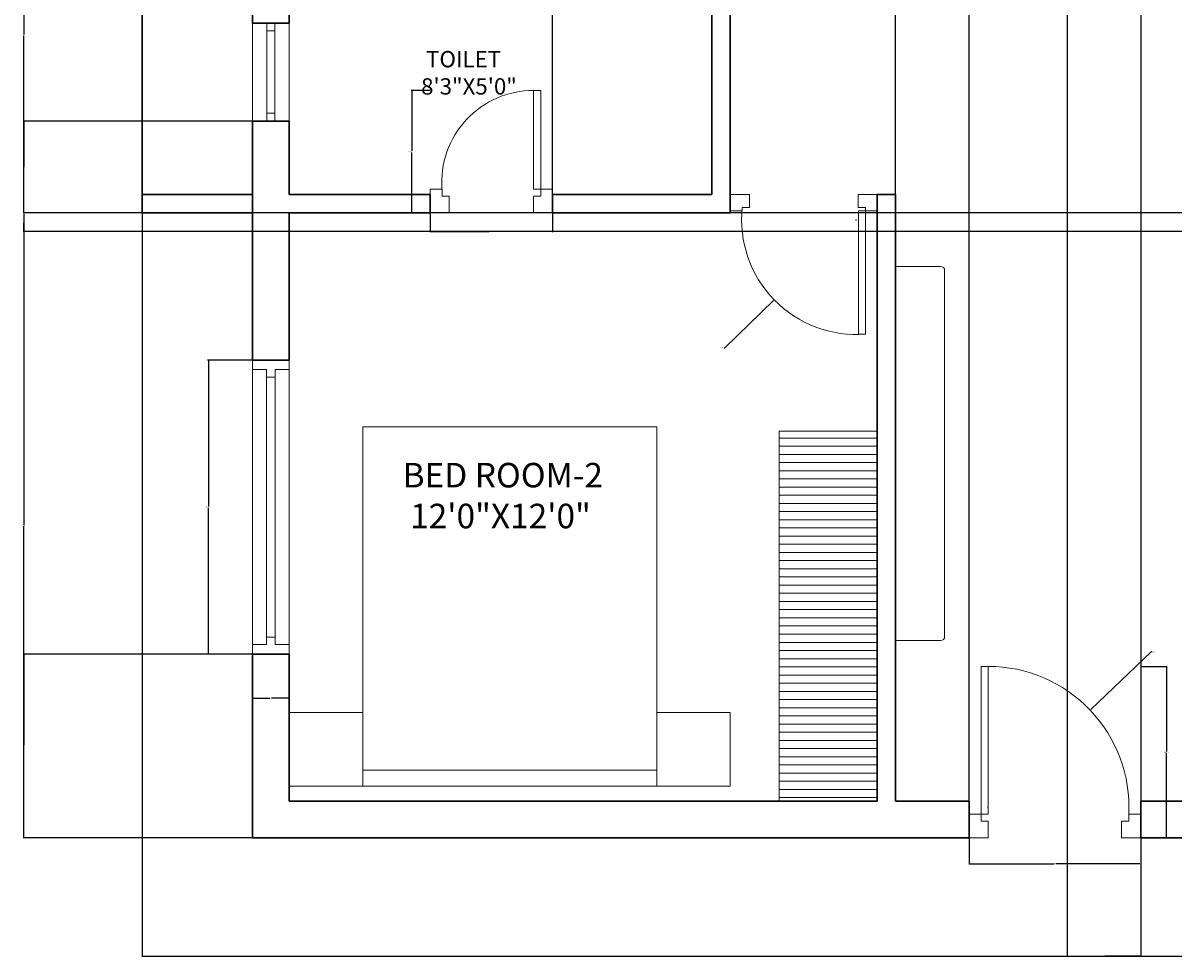
# Model space of a CAD drawing. Units: inches. Extents: x 2134 to 2768, y 715 to 1206.
# Tile 1 of 4: x 2135 to 2416, y 715 to 944. Entities that reach past the tile are written whole.
import ezdxf

# ---------------------------------------------------------------- set-up
doc = ezdxf.new("R2010")
doc.units = ezdxf.units.IN
for name, color, linetype, lineweight in [('A-ANNO-DIMS', 2, 'Continuous', 18), ('A-AREA-IDEN', 7, 'Continuous', 18), ('A-DOOR', 251, 'Continuous', 13), ('A-FLOR-CASE', 251, 'Continuous', 13), ('A-FLOR-CASE-PATT', 252, 'Continuous', 9), ('A-FURN', 251, 'Continuous', 13), ('A-WALL', 7, 'Continuous', 30), ('A-WINDOW', 251, 'Continuous', 13)]:
    doc.layers.add(name, color=color, linetype=linetype, lineweight=lineweight)
doc.styles.get("Standard").update_dxf_attribs({"font": 'arial.ttf'})
doc.dimstyles.get("Standard").update_dxf_attribs({"dimtxt": 0.18, "dimasz": 0.18, "dimexe": 0.18, "dimexo": 0.0625, "dimgap": 0.09, "dimtad": 0, "dimtih": 1, "dimtoh": 1, "dimdec": 4, "dimzin": 0, "dimdsep": 46, "dimtxsty": 'Standard', "dimcen": 0.09, "dimadec": 0, "dimazin": 0, "dimtfac": 1, "dimtdec": 4, "dimtofl": 0, "dimtmove": 0, "dimatfit": 3, "dimfxl": 1, "dimtolj": 1, "dimtzin": 0, "dimarcsym": 0})

# ---------------------------------------------------------------- blocks, each defined once
blk = doc.blocks.new('3 6 2')
at = {"layer": 'A-DOOR'}
for points in [[(-36.75, 5.83), (-36.75, 42), (-35, 42), (-35, 5.83)], [(-36.75, 4.08), (-35, 4.08), (-35, 0), (-39.67, 0), (-39.67, 5.83), (-36.75, 5.83)], [(-0.58, 5.83), (-0.58, 4.08), (-2.33, 4.08), (-2.33, 0), (2.33, 0), (2.33, 5.83)]]:
    blk.add_lwpolyline(points, close=True, dxfattribs=at)
at = {"layer": 'A-DOOR', "ltscale": 0.1}
blk.add_arc((-35, 7.54), 34.46, 357.1595, 90, dxfattribs=at)
blk = doc.blocks.new('ARCHITRAVE')
at = {"layer": 'A-DOOR'}
for p, q in [((0, 0), (0, 4)), ((0, 3.99), (2.92, 3.99)), ((2.92, 3.99), (2.92, 3.17)), ((2.92, 3.17), (4.67, 3.17)), ((4.67, 3.17), (4.67, 0)), ((4.67, 0), (0, 0))]:
    blk.add_line(p, q, dxfattribs=at)
blk = doc.blocks.new('3 FEET DOOR')
at = {"layer": 'A-DOOR'}
blk.add_lwpolyline([(-34.02, 3.98), (-34.02, 34.15), (-32.27, 34.15), (-32.27, 3.98)], close=True, dxfattribs=at)
at = {"layer": 'A-DOOR', "ltscale": 0.1}
blk.add_arc((-31.74, 6.19), 28.05, 353.8214, 94.662, dxfattribs=at)
at = {"layer": 'A-DOOR'}
blk.add_blockref('ARCHITRAVE', (-36.91, 0), dxfattribs=at)
at = {"layer": 'A-DOOR', "xscale": -1}
blk.add_blockref('ARCHITRAVE', (-0.93, 0), dxfattribs=at)
blk = doc.blocks.new('2 feet 6 inch door')
at = {"layer": 'A-DOOR'}
for points in [[(2.92, 5.83), (2.92, 30), (4.67, 30), (4.67, 5.83)], [(2.92, 4.08), (4.67, 4.08), (4.67, 0), (0, 0), (0, 5.83), (2.92, 5.83)], [(27.08, 5.83), (27.08, 4.08), (25.33, 4.08), (25.33, 0), (30, 0), (30, 5.83)]]:
    blk.add_lwpolyline(points, close=True, dxfattribs=at)
at = {"layer": 'A-DOOR', "ltscale": 0.1}
blk.add_arc((4.67, 7.52), 22.48, 355.6972, 90, dxfattribs=at)
blk = doc.blocks.new('bed')
at = {"layer": 'A-FURN'}
for points in [[(3369.68, 925.24), (3297.68, 925.24), (3297.68, 1009.24), (3369.68, 1009.24)], [(3297.68, 921.32), (3279.68, 921.32), (3279.68, 939.32), (3297.68, 939.32)], [(3369.68, 921.32), (3387.68, 921.32), (3387.68, 939.32), (3369.68, 939.32)], [(3297.68, 925.24), (3369.68, 925.24), (3369.68, 921.32), (3297.68, 921.32)]]:
    blk.add_lwpolyline(points, close=True, dxfattribs=at)
blk = doc.blocks.new("2' ventilators")
at = {"layer": 'A-WINDOW'}
for p, q in [((24, 5.5), (0, 5.5)), ((1.93, 5.5), (1.93, 3.5)), ((22.07, 5.5), (22.07, 3.5))]:
    blk.add_line(p, q, dxfattribs=at)
for points in [[(0, 9), (24, 9), (24, 0), (0, 0), (0, 9)], [(24, 3.5), (0, 3.5)]]:
    blk.add_lwpolyline(points, dxfattribs=at)
blk = doc.blocks.new('WINDOW FRAME')
at = {"layer": 'A-WINDOW'}
for points in [[(4178.2, 4970.76), (4174.8, 4970.76), (4174.8, 4968.41), (4183.8, 4968.41), (4183.8, 4970.76), (4180.39, 4970.76)], [(4180.39, 4970.76), (4180.39, 4972.59), (4178.2, 4972.59), (4178.2, 4970.76)]]:
    blk.add_lwpolyline(points, dxfattribs=at)
blk = doc.blocks.new('6 feet door')
at = {"layer": 'A-WINDOW'}
for p, q in [((-69.65, 9), (-2.35, 9)), ((-4.18, 5.59), (-67.82, 5.59)), ((-4.18, 3.41), (-67.82, 3.41)), ((-69.65, 0), (-2.35, 0))]:
    blk.add_line(p, q, dxfattribs=at)
at = {"layer": 'A-WINDOW', "rotation": 270}
blk.add_blockref('WINDOW FRAME', (-5040.41, 4183.8), dxfattribs=at)
at = {"layer": 'A-WINDOW', "xscale": -1, "rotation": 90}
blk.add_blockref('WINDOW FRAME', (4968.41, 4183.8), dxfattribs=at)
blk = doc.blocks.new('*D53')
at = {"layer": 'A-ANNO-DIMS', "color": 0, "lineweight": -2, "transparency": 16777216}
for p, q in [((2234.22, 927.11), (2229.61, 927.11)), ((2229.79, 926.93), (2229.79, 912.29)), ((2229.79, 897.29), (2229.79, 911.92)), ((2234.22, 897.11), (2229.61, 897.11))]:
    blk.add_line(p, q, dxfattribs=at)
at = {"layer": 'A-ANNO-DIMS', "color": 0, "transparency": 16777216}
for points in [[(2229.76, 926.93), (2229.82, 926.93), (2229.79, 927.11)], [(2229.76, 897.29), (2229.82, 897.29), (2229.79, 897.11)]]:
    blk.add_solid(points, dxfattribs=at)
at = {"layer": 'Defpoints', "color": 0, "transparency": 16777216}
for p in [(2229.79, 927.11), (2234.29, 927.11), (2234.29, 897.11)]:
    blk.add_point(p, dxfattribs=at)
at = {"layer": 'A-ANNO-DIMS', "color": 0, "transparency": 16777216, "insert": (2229.79, 912.11), "char_height": 0.18, "attachment_point": 5}
blk.add_mtext('\\A1;BATH DOOR 30 TYP.', dxfattribs=at)
blk = doc.blocks.new('*D54')
at = {"layer": 'A-ANNO-DIMS', "color": 0, "lineweight": -2, "transparency": 16777216}
for p, q in [((2234.29, 897.04), (2234.29, 892.43)), ((2264.29, 897.04), (2264.29, 892.43)), ((2234.47, 892.61), (2248.76, 892.61)), ((2264.11, 892.61), (2249.82, 892.61))]:
    blk.add_line(p, q, dxfattribs=at)
at = {"layer": 'A-ANNO-DIMS', "color": 0, "transparency": 16777216}
for points in [[(2234.47, 892.64), (2234.47, 892.58), (2234.29, 892.61)], [(2264.11, 892.64), (2264.11, 892.58), (2264.29, 892.61)]]:
    blk.add_solid(points, dxfattribs=at)
at = {"layer": 'Defpoints', "color": 0, "transparency": 16777216}
for p in [(2234.29, 897.11), (2264.29, 897.11), (2234.29, 892.61)]:
    blk.add_point(p, dxfattribs=at)
at = {"layer": 'A-ANNO-DIMS', "color": 0, "transparency": 16777216, "insert": (2249.29, 892.61), "char_height": 0.18, "attachment_point": 5}
blk.add_mtext('\\A1;30 TYP.', dxfattribs=at)
blk = doc.blocks.new('*D69')
at = {"layer": 'A-ANNO-DIMS', "color": 0, "lineweight": -2, "transparency": 16777216}
for p, q in [((2408.35, 786.11), (2414.77, 786.11)), ((2414.59, 785.93), (2414.59, 765.29)), ((2414.59, 744.29), (2414.59, 764.93)), ((2408.35, 744.11), (2414.77, 744.11))]:
    blk.add_line(p, q, dxfattribs=at)
at = {"layer": 'A-ANNO-DIMS', "color": 0, "transparency": 16777216}
for points in [[(2414.56, 785.93), (2414.62, 785.93), (2414.59, 786.11)], [(2414.56, 744.29), (2414.62, 744.29), (2414.59, 744.11)]]:
    blk.add_solid(points, dxfattribs=at)
at = {"layer": 'Defpoints', "color": 0, "transparency": 16777216}
for p in [(2408.29, 786.11), (2414.59, 786.11), (2408.29, 744.11)]:
    blk.add_point(p, dxfattribs=at)
at = {"layer": 'A-ANNO-DIMS', "color": 0, "transparency": 16777216, "insert": (2414.59, 765.11), "char_height": 0.18, "attachment_point": 5}
blk.add_mtext('\\A1;ENTRY 42', dxfattribs=at)
blk = doc.blocks.new('*D70')
at = {"layer": 'A-ANNO-DIMS', "color": 0, "lineweight": -2, "transparency": 16777216}
for p, q in [((2366.29, 744.04), (2366.29, 737.63)), ((2408.29, 744.04), (2408.29, 737.63)), ((2366.47, 737.81), (2387.07, 737.81)), ((2408.11, 737.81), (2387.51, 737.81))]:
    blk.add_line(p, q, dxfattribs=at)
at = {"layer": 'A-ANNO-DIMS', "color": 0, "transparency": 16777216}
for points in [[(2366.47, 737.84), (2366.47, 737.78), (2366.29, 737.81)], [(2408.11, 737.84), (2408.11, 737.78), (2408.29, 737.81)]]:
    blk.add_solid(points, dxfattribs=at)
at = {"layer": 'Defpoints', "color": 0, "transparency": 16777216}
for p in [(2366.29, 744.11), (2408.29, 744.11), (2408.29, 737.81)]:
    blk.add_point(p, dxfattribs=at)
at = {"layer": 'A-ANNO-DIMS', "color": 0, "transparency": 16777216, "insert": (2387.29, 737.81), "char_height": 0.18, "attachment_point": 5}
blk.add_mtext('\\A1;42', dxfattribs=at)
blk = doc.blocks.new('*D73')
at = {"layer": 'A-ANNO-DIMS', "color": 0, "lineweight": -2, "transparency": 16777216}
for p, q in [((2190.72, 861.11), (2179.81, 861.11)), ((2179.99, 860.93), (2179.99, 825.29)), ((2179.99, 789.29), (2179.99, 824.92)), ((2190.72, 789.11), (2179.81, 789.11))]:
    blk.add_line(p, q, dxfattribs=at)
at = {"layer": 'A-ANNO-DIMS', "color": 0, "transparency": 16777216}
for points in [[(2179.96, 860.93), (2180.02, 860.93), (2179.99, 861.11)], [(2179.96, 789.29), (2180.02, 789.29), (2179.99, 789.11)]]:
    blk.add_solid(points, dxfattribs=at)
at = {"layer": 'Defpoints', "color": 0, "transparency": 16777216}
for p in [(2190.79, 861.11), (2179.99, 789.11), (2190.79, 789.11)]:
    blk.add_point(p, dxfattribs=at)
at = {"layer": 'A-ANNO-DIMS', "color": 0, "transparency": 16777216, "insert": (2179.99, 825.11), "char_height": 0.18, "attachment_point": 5}
blk.add_mtext('\\A1;GLAZING 72', dxfattribs=at)
blk = doc.blocks.new('*D74')
at = {"layer": 'A-ANNO-DIMS', "color": 0, "lineweight": -2, "transparency": 16777216}
for p, q in [((2190.79, 789.04), (2190.79, 778.13)), ((2199.79, 789.04), (2199.79, 778.13)), ((2190.97, 778.31), (2195.14, 778.31)), ((2199.61, 778.31), (2195.44, 778.31))]:
    blk.add_line(p, q, dxfattribs=at)
at = {"layer": 'A-ANNO-DIMS', "color": 0, "transparency": 16777216}
for points in [[(2190.97, 778.34), (2190.97, 778.28), (2190.79, 778.31)], [(2199.61, 778.34), (2199.61, 778.28), (2199.79, 778.31)]]:
    blk.add_solid(points, dxfattribs=at)
at = {"layer": 'Defpoints', "color": 0, "transparency": 16777216}
for p in [(2190.79, 789.11), (2199.79, 789.11), (2199.79, 778.31)]:
    blk.add_point(p, dxfattribs=at)
at = {"layer": 'A-ANNO-DIMS', "color": 0, "transparency": 16777216, "insert": (2195.29, 778.31), "char_height": 0.18, "attachment_point": 5}
blk.add_mtext('\\A1;9', dxfattribs=at)
blk = doc.blocks.new('*D81')
at = {"layer": 'A-ANNO-DIMS', "color": 0, "lineweight": -2, "transparency": 16777216}
for p, q in [((2163.72, 897.11), (2134.66, 897.11)), ((2134.84, 896.93), (2134.84, 820.79)), ((2134.84, 744.29), (2134.84, 820.43)), ((2190.72, 744.11), (2134.66, 744.11))]:
    blk.add_line(p, q, dxfattribs=at)
at = {"layer": 'A-ANNO-DIMS', "color": 0, "transparency": 16777216}
for points in [[(2134.81, 896.93), (2134.87, 896.93), (2134.84, 897.11)], [(2134.81, 744.29), (2134.87, 744.29), (2134.84, 744.11)]]:
    blk.add_solid(points, dxfattribs=at)
at = {"layer": 'Defpoints', "color": 0, "transparency": 16777216}
for p in [(2134.84, 897.11), (2163.79, 897.11), (2190.79, 744.11)]:
    blk.add_point(p, dxfattribs=at)
at = {"layer": 'A-ANNO-DIMS', "color": 0, "transparency": 16777216, "insert": (2134.84, 820.61), "char_height": 0.18, "attachment_point": 5}
blk.add_mtext('\\A1;153', dxfattribs=at)
blk = doc.blocks.new('*D82')
at = {"layer": 'A-ANNO-DIMS', "color": 0, "lineweight": -2, "transparency": 16777216}
for p, q in [((2163.72, 984.11), (2134.66, 984.11)), ((2134.84, 983.93), (2134.84, 940.79)), ((2134.84, 897.29), (2134.84, 940.43)), ((2163.72, 897.11), (2134.66, 897.11))]:
    blk.add_line(p, q, dxfattribs=at)
at = {"layer": 'A-ANNO-DIMS', "color": 0, "transparency": 16777216}
for points in [[(2134.81, 983.93), (2134.87, 983.93), (2134.84, 984.11)], [(2134.81, 897.29), (2134.87, 897.29), (2134.84, 897.11)]]:
    blk.add_solid(points, dxfattribs=at)
at = {"layer": 'Defpoints', "color": 0, "transparency": 16777216}
for p in [(2134.84, 984.11), (2163.79, 984.11), (2163.79, 897.11)]:
    blk.add_point(p, dxfattribs=at)
at = {"layer": 'A-ANNO-DIMS', "color": 0, "transparency": 16777216, "insert": (2134.84, 940.61), "char_height": 0.18, "attachment_point": 5}
blk.add_mtext('\\A1;87', dxfattribs=at)
blk = doc.blocks.new('*D83')
at = {"layer": 'A-ANNO-DIMS', "color": 0, "lineweight": -2, "transparency": 16777216}
for p, q in [((2348.29, 753.17), (2348.29, 1205.74)), ((2348.47, 1205.56), (2357.08, 1205.56)), ((2366.11, 1205.56), (2357.5, 1205.56)), ((2366.29, 753.17), (2366.29, 1205.74))]:
    blk.add_line(p, q, dxfattribs=at)
at = {"layer": 'A-ANNO-DIMS', "color": 0, "transparency": 16777216}
for points in [[(2348.47, 1205.59), (2348.47, 1205.53), (2348.29, 1205.56)], [(2366.11, 1205.59), (2366.11, 1205.53), (2366.29, 1205.56)]]:
    blk.add_solid(points, dxfattribs=at)
at = {"layer": 'Defpoints', "color": 0, "transparency": 16777216}
for p in [(2366.29, 1205.56), (2348.29, 753.11), (2366.29, 753.11)]:
    blk.add_point(p, dxfattribs=at)
at = {"layer": 'A-ANNO-DIMS', "color": 0, "transparency": 16777216, "insert": (2357.29, 1205.56), "char_height": 0.18, "attachment_point": 5}
blk.add_mtext('\\A1;18', dxfattribs=at)
blk = doc.blocks.new('*D86')
at = {"layer": 'A-ANNO-DIMS', "color": 0, "lineweight": -2, "transparency": 16777216}
for p, q in [((2190.72, 789.11), (2134.66, 789.11)), ((2134.84, 788.93), (2134.84, 766.79)), ((2134.84, 744.29), (2134.84, 766.43)), ((2190.72, 744.11), (2134.66, 744.11))]:
    blk.add_line(p, q, dxfattribs=at)
at = {"layer": 'A-ANNO-DIMS', "color": 0, "transparency": 16777216}
for points in [[(2134.81, 788.93), (2134.87, 788.93), (2134.84, 789.11)], [(2134.81, 744.29), (2134.87, 744.29), (2134.84, 744.11)]]:
    blk.add_solid(points, dxfattribs=at)
at = {"layer": 'Defpoints', "color": 0, "transparency": 16777216}
for p in [(2134.84, 789.11), (2190.79, 789.11), (2190.79, 744.11)]:
    blk.add_point(p, dxfattribs=at)
at = {"layer": 'A-ANNO-DIMS', "color": 0, "transparency": 16777216, "insert": (2134.84, 766.61), "char_height": 0.18, "attachment_point": 5}
blk.add_mtext('\\A1;45', dxfattribs=at)
blk = doc.blocks.new('*D88')
at = {"layer": 'A-ANNO-DIMS', "color": 0, "lineweight": -2, "transparency": 16777216}
for p, q in [((2190.72, 919.61), (2134.66, 919.61)), ((2134.84, 919.43), (2134.84, 908.54)), ((2134.84, 897.29), (2134.84, 908.18)), ((2190.72, 897.11), (2134.66, 897.11))]:
    blk.add_line(p, q, dxfattribs=at)
at = {"layer": 'A-ANNO-DIMS', "color": 0, "transparency": 16777216}
for points in [[(2134.81, 919.43), (2134.87, 919.43), (2134.84, 919.61)], [(2134.81, 897.29), (2134.87, 897.29), (2134.84, 897.11)]]:
    blk.add_solid(points, dxfattribs=at)
at = {"layer": 'Defpoints', "color": 0, "transparency": 16777216}
for p in [(2134.84, 919.61), (2190.79, 919.61), (2190.79, 897.11)]:
    blk.add_point(p, dxfattribs=at)
at = {"layer": 'A-ANNO-DIMS', "color": 0, "transparency": 16777216, "insert": (2134.84, 908.36), "char_height": 0.18, "attachment_point": 5}
blk.add_mtext('\\A1;22.5', dxfattribs=at)
blk = doc.blocks.new('*D90')
at = {"layer": 'A-ANNO-DIMS', "color": 0, "lineweight": -2, "transparency": 16777216}
for p, q in [((2729.72, 897.11), (2134.66, 897.11)), ((2134.84, 896.93), (2134.84, 895.04)), ((2134.84, 892.79), (2134.84, 894.68)), ((2729.72, 892.61), (2134.66, 892.61))]:
    blk.add_line(p, q, dxfattribs=at)
at = {"layer": 'A-ANNO-DIMS', "color": 0, "transparency": 16777216}
for points in [[(2134.81, 896.93), (2134.87, 896.93), (2134.84, 897.11)], [(2134.81, 892.79), (2134.87, 892.79), (2134.84, 892.61)]]:
    blk.add_solid(points, dxfattribs=at)
at = {"layer": 'Defpoints', "color": 0, "transparency": 16777216}
for p in [(2729.79, 897.11), (2134.84, 892.61), (2729.79, 892.61)]:
    blk.add_point(p, dxfattribs=at)
at = {"layer": 'A-ANNO-DIMS', "color": 0, "transparency": 16777216, "insert": (2134.84, 894.86), "char_height": 0.18, "attachment_point": 5}
blk.add_mtext('\\A1;4.5', dxfattribs=at)
blk = doc.blocks.new('*D91')
at = {"layer": 'A-ANNO-DIMS', "color": 0, "lineweight": -2, "transparency": 16777216}
for p, q in [((2390.29, 1115.04), (2390.29, 714.98)), ((2408.29, 1115.04), (2408.29, 714.98)), ((2390.47, 715.16), (2399.08, 715.16)), ((2408.11, 715.16), (2399.5, 715.16))]:
    blk.add_line(p, q, dxfattribs=at)
at = {"layer": 'A-ANNO-DIMS', "color": 0, "transparency": 16777216}
for points in [[(2390.47, 715.19), (2390.47, 715.13), (2390.29, 715.16)], [(2408.11, 715.19), (2408.11, 715.13), (2408.29, 715.16)]]:
    blk.add_solid(points, dxfattribs=at)
at = {"layer": 'Defpoints', "color": 0, "transparency": 16777216}
for p in [(2390.29, 1115.11), (2408.29, 1115.11), (2408.29, 715.16)]:
    blk.add_point(p, dxfattribs=at)
at = {"layer": 'A-ANNO-DIMS', "color": 0, "transparency": 16777216, "insert": (2399.29, 715.16), "char_height": 0.18, "attachment_point": 5}
blk.add_mtext('\\A1;18', dxfattribs=at)
blk = doc.blocks.new('*D103')
at = {"layer": 'A-ANNO-DIMS', "color": 0, "lineweight": -2, "transparency": 16777216}
for p, q in [((2264.29, 901.67), (2264.29, 1205.74)), ((2264.47, 1205.56), (2283.57, 1205.56)), ((2303.11, 1205.56), (2284.01, 1205.56)), ((2303.29, 901.67), (2303.29, 1205.74))]:
    blk.add_line(p, q, dxfattribs=at)
at = {"layer": 'A-ANNO-DIMS', "color": 0, "transparency": 16777216}
for points in [[(2264.47, 1205.59), (2264.47, 1205.53), (2264.29, 1205.56)], [(2303.11, 1205.59), (2303.11, 1205.53), (2303.29, 1205.56)]]:
    blk.add_solid(points, dxfattribs=at)
at = {"layer": 'Defpoints', "color": 0, "transparency": 16777216}
for p in [(2303.29, 1205.56), (2264.29, 901.61), (2303.29, 901.61)]:
    blk.add_point(p, dxfattribs=at)
at = {"layer": 'A-ANNO-DIMS', "color": 0, "transparency": 16777216, "insert": (2283.79, 1205.56), "char_height": 0.18, "attachment_point": 5}
blk.add_mtext('\\A1;39', dxfattribs=at)
blk = doc.blocks.new('*D105')
at = {"layer": 'A-ANNO-DIMS', "color": 0, "lineweight": -2, "transparency": 16777216}
for p, q in [((2163.79, 897.04), (2163.79, 714.98)), ((2738.79, 744.04), (2738.79, 714.98)), ((2163.97, 715.16), (2451, 715.16)), ((2738.61, 715.16), (2451.58, 715.16))]:
    blk.add_line(p, q, dxfattribs=at)
at = {"layer": 'A-ANNO-DIMS', "color": 0, "transparency": 16777216}
for points in [[(2163.97, 715.19), (2163.97, 715.13), (2163.79, 715.16)], [(2738.61, 715.19), (2738.61, 715.13), (2738.79, 715.16)]]:
    blk.add_solid(points, dxfattribs=at)
at = {"layer": 'Defpoints', "color": 0, "transparency": 16777216}
for p in [(2163.79, 897.11), (2738.79, 744.11), (2738.79, 715.16)]:
    blk.add_point(p, dxfattribs=at)
at = {"layer": 'A-ANNO-DIMS', "color": 0, "transparency": 16777216, "insert": (2451.29, 715.16), "char_height": 0.18, "attachment_point": 5}
blk.add_mtext('\\A1;575', dxfattribs=at)
blk = doc.blocks.new('*D107')
at = {"layer": 'A-ANNO-DIMS', "color": 0, "lineweight": -2, "transparency": 16777216}
for p, q in [((2410.89, 789.66), (2396.05, 775.53)), ((2411.07, 789.66), (2410.89, 789.66)), ((2370.86, 751.65), (2371.04, 751.65)), ((2370.95, 751.56), (2370.95, 751.74))]:
    blk.add_line(p, q, dxfattribs=at)
at = {"layer": 'A-ANNO-DIMS', "color": 0, "transparency": 16777216}
blk.add_solid([(2396.03, 775.55), (2396.07, 775.51), (2395.92, 775.4)], dxfattribs=at)
at = {"layer": 'Defpoints', "color": 0, "transparency": 16777216}
for p in [(2395.92, 775.4), (2370.95, 751.65)]:
    blk.add_point(p, dxfattribs=at)
at = {"layer": 'A-ANNO-DIMS', "color": 0, "transparency": 16777216, "insert": (2411.55, 789.66), "char_height": 0.18, "attachment_point": 5}
blk.add_mtext('\\A1;R34.46', dxfattribs=at)
blk = doc.blocks.new('*D108')
at = {"layer": 'A-ANNO-DIMS', "color": 0, "lineweight": -2, "transparency": 16777216}
for p, q in [((2338.62, 895.33), (2338.62, 895.51)), ((2338.53, 895.42), (2338.71, 895.42)), ((2306.47, 864.1), (2318.39, 875.72)), ((2306.29, 864.1), (2306.47, 864.1))]:
    blk.add_line(p, q, dxfattribs=at)
at = {"layer": 'A-ANNO-DIMS', "color": 0, "transparency": 16777216}
blk.add_solid([(2318.37, 875.74), (2318.42, 875.7), (2318.52, 875.85)], dxfattribs=at)
at = {"layer": 'Defpoints', "color": 0, "transparency": 16777216}
for p in [(2338.62, 895.42), (2318.52, 875.85)]:
    blk.add_point(p, dxfattribs=at)
at = {"layer": 'A-ANNO-DIMS', "color": 0, "transparency": 16777216, "insert": (2305.81, 864.1), "char_height": 0.18, "attachment_point": 5}
blk.add_mtext('\\A1;R28.05', dxfattribs=at)

msp = doc.modelspace()

# ---------------------------------------------------------------- hatches: boundary and pattern name
at = {"layer": 'A-FLOR-CASE-PATT'}
h = msp.add_hatch(dxfattribs=at)
h.set_pattern_fill('_USER', color=256, scale=2, pattern_type=0)
h.set_pattern_definition([(0, (0, 0), (0, 2), [])])
h.paths.add_polyline_path([(2343.787, 843.68), (2319.787, 843.68), (2319.787, 753.107), (2343.787, 753.107)])

# ---------------------------------------------------------------- linework, layer by layer
at = {"layer": 'A-FLOR-CASE'}
for p, q in [((2348.287, 884.029), (2359.287, 884.029)), ((2360.287, 883.029), (2360.287, 793.422)), ((2319.787, 843.68), (2319.787, 753.107)), ((2319.787, 843.68), (2343.787, 843.68)), ((2359.287, 792.422), (2348.287, 792.422))]:
    msp.add_line(p, q, dxfattribs=at)
for centre, start, end in [((2359.287, 883.029), 0, 90), ((2359.287, 793.422), 270, 0)]:
    msp.add_arc(centre, 1, start, end, dxfattribs=at)
at = {"layer": 'A-WALL'}
for p, q in [((2163.787, 979.607), (2163.787, 901.607)), ((2190.787, 979.607), (2190.787, 943.607)), ((2307.787, 966.107), (2307.787, 897.107)), ((2199.787, 961.607), (2199.787, 943.607)), ((2303.287, 961.607), (2303.287, 901.607)), ((2199.787, 943.607), (2190.787, 943.607)), ((2199.787, 919.607), (2190.787, 919.607)), ((2190.787, 919.607), (2190.787, 861.107)), ((2199.787, 919.607), (2199.787, 901.607)), ((2163.787, 897.107), (2163.787, 901.607)), ((2190.787, 901.607), (2163.787, 901.607)), ((2234.287, 901.607), (2199.787, 901.607)), ((2234.287, 901.607), (2234.287, 897.107)), ((2303.287, 901.607), (2264.287, 901.607)), ((2264.287, 901.607), (2264.287, 897.107)), ((2343.787, 901.607), (2348.287, 901.607)), ((2343.787, 901.607), (2343.787, 753.107)), ((2348.287, 901.607), (2348.287, 753.107)), ((2190.787, 897.107), (2163.787, 897.107)), ((2234.287, 897.107), (2199.787, 897.107)), ((2199.787, 897.107), (2199.787, 861.107)), ((2307.787, 897.107), (2264.287, 897.107)), ((2199.787, 861.107), (2190.787, 861.107)), ((2199.787, 789.107), (2190.787, 789.107)), ((2190.787, 789.107), (2190.787, 744.107)), ((2199.787, 789.107), (2199.787, 753.107)), ((2343.787, 753.107), (2199.787, 753.107)), ((2366.287, 753.107), (2348.287, 753.107)), ((2366.287, 753.107), (2366.287, 744.107)), ((2408.287, 753.107), (2408.287, 744.107)), ((2467.287, 753.107), (2408.287, 753.107)), ((2366.287, 744.107), (2190.787, 744.107)), ((2467.287, 744.107), (2408.287, 744.107))]:
    msp.add_line(p, q, dxfattribs=at)

# ---------------------------------------------------------------- block references
at = {"layer": 'A-DOOR', "xscale": -1}
msp.add_blockref('2 feet 6 inch door', (2264.287, 897.107), dxfattribs=at)
at = {"layer": 'A-DOOR', "rotation": 180}
msp.add_blockref('3 FEET DOOR', (2306.88, 901.607), dxfattribs=at)
at = {"layer": 'A-DOOR'}
msp.add_blockref('3 6 2', (2405.954, 744.107), dxfattribs=at)
at = {"layer": 'A-FURN'}
msp.add_blockref('bed', (-1079.895, -164.514), dxfattribs=at)
at = {"layer": 'A-WINDOW'}
for name, p, rotation in [("2' ventilators", (2190.787, 943.607), 270), ('6 feet door', (2190.787, 789.107), 270.000009980655)]:
    msp.add_blockref(name, p, dxfattribs=dict(at, rotation=rotation))

# ---------------------------------------------------------------- texts
at = {"layer": 'A-AREA-IDEN', "attachment_point": 1}
for s, insert, char_height in [('  TOILET\\P 8\'3"X5\'0"', (2230.859, 936.756), 4), ('BED ROOM-2\\P 12\'0"X12\'0"', (2227.563, 835.925), 6)]:
    msp.add_mtext_dynamic_manual_height_columns(s, width=55.72169, gutter_width=12.5, heights=[0], dxfattribs=dict(at, insert=insert, char_height=char_height))

# ---------------------------------------------------------------- dimensions: what is measured, and where the dimension line sits
at = {"layer": 'A-ANNO-DIMS'}
for base, p1, p2, picture, middle in [((2303.287, 1205.557), (2264.287, 901.607), (2303.287, 901.607), '*D103', (2283.787, 1205.557)), ((2366.287, 1205.557), (2348.287, 753.107), (2366.287, 753.107), '*D83', (2357.287, 1205.557)), ((2408.287, 715.157), (2390.287, 1115.107), (2408.287, 1115.107), '*D91', (2399.287, 715.157)), ((2738.787, 715.157), (2163.787, 897.107), (2738.787, 744.107), '*D105', (2451.287, 715.157)), ((2408.287, 737.807), (2366.287, 744.107), (2408.287, 744.107), '*D70', (2387.287, 737.807))]:
    dim = msp.add_linear_dim(base=base, p1=p1, p2=p2, dimstyle='Standard', override={"dimdec": 0, "dimlfac": 1, "dimrnd": 0, "dimzin": 0, "dimdsep": 46, "dimlunit": 2}, dxfattribs=at)
    dim.commit()
    dim.dimension.update_dxf_attribs({"geometry": picture, "text_midpoint": middle})
for base, p1, p2, angle, override, picture, middle in [((2134.837, 984.107), (2163.787, 897.107), (2163.787, 984.107), 90, {"dimdec": 0, "dimlfac": 1, "dimrnd": 0, "dimzin": 0, "dimdsep": 46, "dimlunit": 2}, '*D82', (2134.837, 940.607)), ((2134.837, 919.607), (2190.787, 897.107), (2190.787, 919.607), 90, {"dimdec": 1, "dimlfac": 1, "dimrnd": 0, "dimzin": 0, "dimdsep": 46, "dimlunit": 2}, '*D88', (2134.837, 908.357)), ((2134.837, 897.107), (2190.787, 744.107), (2163.787, 897.107), 90, {"dimdec": 0, "dimlfac": 1, "dimrnd": 0, "dimzin": 0, "dimdsep": 46, "dimlunit": 2}, '*D81', (2134.837, 820.607)), ((2134.837, 892.607), (2729.787, 897.107), (2729.787, 892.607), 90, {"dimdec": 1, "dimlfac": 1, "dimrnd": 0, "dimzin": 0, "dimdsep": 46, "dimlunit": 2}, '*D90', (2134.837, 894.857)), ((2134.837, 789.107), (2190.787, 744.107), (2190.787, 789.107), 90, {"dimdec": 0, "dimlfac": 1, "dimrnd": 0, "dimzin": 0, "dimdsep": 46, "dimlunit": 2}, '*D86', (2134.837, 766.607)), ((2199.787, 778.307), (2190.787, 789.107), (2199.787, 789.107), 0.00001, {"dimdec": 0, "dimlfac": 1, "dimrnd": 0, "dimzin": 0, "dimdsep": 46, "dimlunit": 2}, '*D74', (2195.287, 778.307))]:
    dim = msp.add_linear_dim(base=base, p1=p1, p2=p2, angle=angle, dimstyle='Standard', override=override, dxfattribs=at)
    dim.commit()
    dim.dimension.update_dxf_attribs({"geometry": picture, "text_midpoint": middle})
for base, p1, p2, angle, text, picture, middle in [((2229.787, 927.107), (2234.287, 897.107), (2234.287, 927.107), 90, 'BATH DOOR <> TYP.', '*D53', (2229.787, 912.107)), ((2234.287, 892.607), (2264.287, 897.107), (2234.287, 897.107), 180, '<> TYP.', '*D54', (2249.287, 892.607)), ((2179.987, 789.107), (2190.787, 861.107), (2190.787, 789.107), 270.00001, 'GLAZING <>', '*D73', (2179.987, 825.107)), ((2414.587, 786.107), (2408.287, 744.107), (2408.287, 786.107), 90, 'ENTRY <>', '*D69', (2414.587, 765.107))]:
    dim = msp.add_linear_dim(base=base, p1=p1, p2=p2, angle=angle, text=text, dimstyle='Standard', override={"dimdec": 0, "dimlfac": 1, "dimrnd": 0, "dimzin": 0, "dimdsep": 46, "dimlunit": 2}, dxfattribs=at)
    dim.commit()
    dim.dimension.update_dxf_attribs({"geometry": picture, "text_midpoint": middle})
for center, mpoint, picture, middle in [((2338.618, 895.417), (2318.523, 875.847), '*D108', (2305.806, 864.105)), ((2370.954, 751.648), (2395.917, 775.403), '*D107', (2411.554, 789.656))]:
    dim = msp.add_radius_dim(center=center, mpoint=mpoint, dimstyle='Standard', override={"dimdec": 2, "dimlfac": 1, "dimrnd": 0, "dimzin": 0, "dimdsep": 46, "dimlunit": 2}, dxfattribs=at)
    dim.commit()
    dim.dimension.update_dxf_attribs({"geometry": picture, "text_midpoint": middle, "dimtype": 164})

doc.saveas('drawing.dxf')
